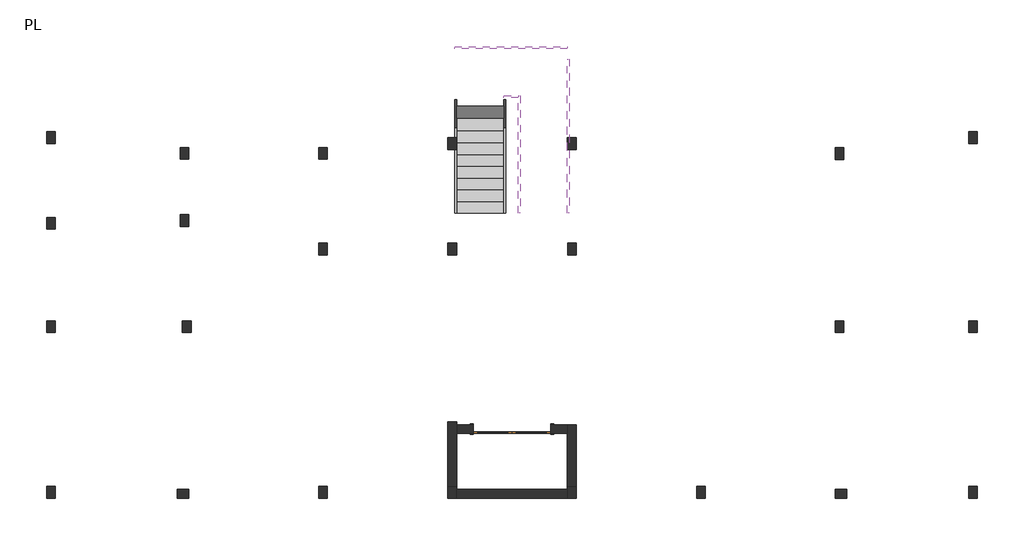
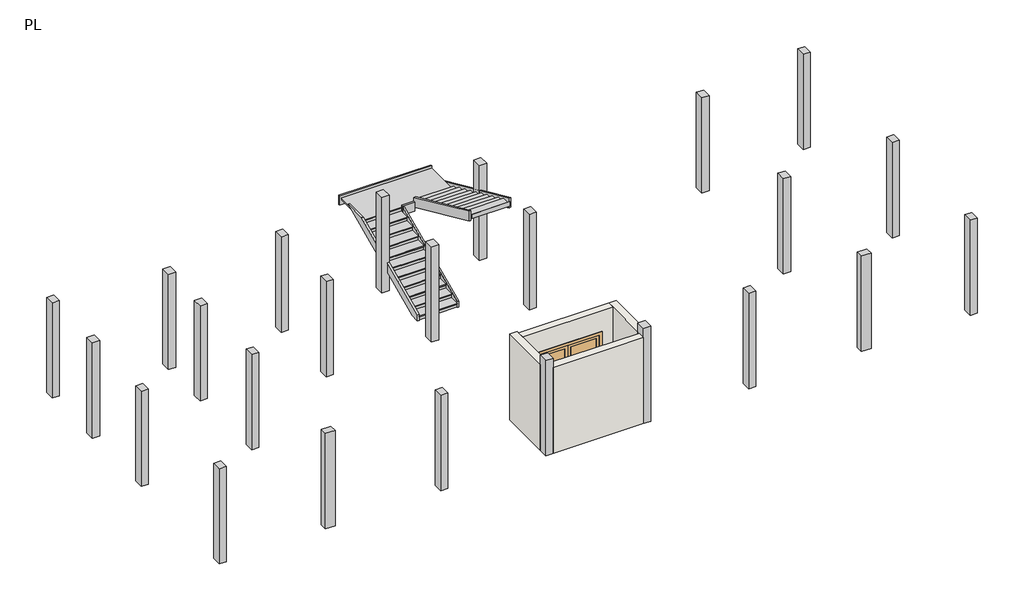
# One storey, incomplete: 24 columns, 6 members, 4 walls, 1 door, 1 stair flight.
"""IFC4 building model written with IfcOpenShell, lengths in millimetres."""

from ifc_helpers import new_model, si_unit, frame, origin, origin_with_axes, place, context, project, spatial, polyline, outline, extrude, faceted_brep, transform, mapped, element, save
from components import column_f87144f2, door_77e2dd85, stair_flight_185d1b01

model = new_model("IFC4")

# Units and contexts
model_context = context("Model", 3, world=origin())
ifc_project = project(units=[si_unit("LENGTHUNIT", "METRE", prefix="MILLI")], contexts=[model_context])

# Site, building, storey
site = spatial("IfcSite", under=ifc_project)
building = spatial("IfcBuilding", under=site)
storey = spatial("IfcBuildingStorey", under=building, Name="PL", Elevation=0.0)

# Columns
placement = place(None, origin())
element("IfcColumn", 1, ObjectType="Rectangular Column : 1'X 9\"", at=placement, inside=storey, context=model_context, shape_type="SweptSolid", body=[
    extrude(outline(polyline([(-12224.6987957, -3709.2932671), (-12224.6987957, -4014.0932671), (-12453.2987957, -4014.0932671), (-12453.2987957, -3709.2932671), (-12224.6987957, -3709.2932671)])), origin_with_axes(), (0.0, 0.0, 1.0), 3200.4),
])
element("IfcColumn", 2, ObjectType="Rectangular Column : 1'X 9\"", at=placement, inside=storey, context=model_context, shape_type="SweptSolid", body=[
    extrude(outline(polyline([(-12224.6987957, 583.3067334), (-12224.6987957, 278.5067334), (-12453.2987957, 278.5067334), (-12453.2987957, 583.3067334), (-12224.6987957, 583.3067334)])), origin_with_axes(), (0.0, 0.0, 1.0), 3200.4),
])
element("IfcColumn", 3, ObjectType="Rectangular Column : 1'X 9\"", at=placement, inside=storey, context=model_context, shape_type="SweptSolid", body=[
    extrude(outline(polyline([(-12224.6987957, 3256.6567332), (-12224.6987957, 2951.8567332), (-12453.2987957, 2951.8567332), (-12453.2987957, 3256.6567332), (-12224.6987957, 3256.6567332)])), origin_with_axes(), (0.0, 0.0, 1.0), 3200.4),
])
element("IfcColumn", 4, ObjectType="Rectangular Column : 1'X 9\"", at=placement, inside=storey, context=model_context, shape_type="SweptSolid", body=[
    extrude(outline(polyline([(-8770.2987992, 5066.406733), (-8770.2987992, 4761.606733), (-8998.8987992, 4761.606733), (-8998.8987992, 5066.406733), (-8770.2987992, 5066.406733)])), origin_with_axes(), (0.0, 0.0, 1.0), 3200.4),
])
element("IfcColumn", 5, ObjectType="Rectangular Column : 1'X 9\"", at=placement, inside=storey, context=model_context, shape_type="SweptSolid", body=[
    extrude(outline(polyline([(-8770.2987992, 3326.5067332), (-8770.2987992, 3021.7067332), (-8998.8987992, 3021.7067332), (-8998.8987992, 3326.5067332), (-8770.2987992, 3326.5067332)])), origin_with_axes(), (0.0, 0.0, 1.0), 3200.4),
])
element("IfcColumn", 6, ObjectType="Rectangular Column : 1'X 9\"", at=placement, inside=storey, context=model_context, shape_type="SweptSolid", body=[
    extrude(outline(polyline([(-8713.148796, 583.3067334), (-8713.148796, 278.5067334), (-8941.748796, 278.5067334), (-8941.748796, 583.3067334), (-8713.148796, 583.3067334)])), origin_with_axes(), (0.0, 0.0, 1.0), 3200.4),
])
element("IfcColumn", 7, ObjectType="Rectangular Column : 1'X 9\"", at=placement, inside=storey, context=model_context, shape_type="SweptSolid", body=[
    extrude(outline(polyline([(-5188.8987995, 5066.406733), (-5188.8987995, 4761.606733), (-5417.4987995, 4761.606733), (-5417.4987995, 5066.406733), (-5188.8987995, 5066.406733)])), origin_with_axes(), (0.0, 0.0, 1.0), 3200.4),
])
element("IfcColumn", 8, ObjectType="Rectangular Column : 1'X 9\"", at=placement, inside=storey, context=model_context, shape_type="SweptSolid", body=[
    extrude(outline(polyline([(-5188.8987995, 2589.9067802), (-5188.8987995, 2285.1067802), (-5417.4987995, 2285.1067802), (-5417.4987995, 2589.9067802), (-5188.8987995, 2589.9067802)])), origin_with_axes(), (0.0, 0.0, 1.0), 3200.4),
])
element("IfcColumn", 9, ObjectType="Rectangular Column : 1'X 9\"", at=placement, inside=storey, context=model_context, shape_type="SweptSolid", body=[
    extrude(outline(polyline([(-5188.8987963, -3709.2932193), (-5188.8987963, -4014.0932193), (-5417.4987963, -4014.0932193), (-5417.4987963, -3709.2932193), (-5188.8987963, -3709.2932193)])), origin_with_axes(), (0.0, 0.0, 1.0), 3200.4),
])
element("IfcColumn", 10, ObjectType="Rectangular Column : 1'X 9\"", at=placement, inside=storey, context=model_context, shape_type="Brep", body=[
    faceted_brep([(1250.0012085, -3709.2932193, 0.0), (1250.0012085, -4014.0932193, 0.0), (1021.4012085, -4014.0932193, 0.0), (1021.4012085, -3785.4932663, 0.0), (1021.4012085, -3709.2932193, 0.0), (1250.0012085, -3709.2932193, 3200.4), (1250.0012085, -4014.0932193, 3200.4), (1250.0012085, -3709.2932193, 2895.6), (1021.4012085, -4014.0932193, 3200.4), (1021.4012085, -3709.2932193, 3200.4), (1021.4012085, -3709.2932193, 2895.6)], [[[0, 1, 2, 3, 4]], [[5, 6, 1, 0, 7]], [[6, 8, 2, 1]], [[8, 9, 10, 4, 3, 2]], [[9, 5, 7, 0, 4, 10]], [[5, 9, 8, 6]]]),
])
element("IfcColumn", 11, ObjectType="Rectangular Column : 1'X 9\"", at=placement, inside=storey, context=model_context, shape_type="SweptSolid", body=[
    extrude(outline(polyline([(4590.1012082, -3709.2932193), (4590.1012082, -4014.0932193), (4361.5012082, -4014.0932193), (4361.5012082, -3709.2932193), (4590.1012082, -3709.2932193)])), origin_with_axes(), (0.0, 0.0, 1.0), 3200.4),
])
element("IfcColumn", 12, ObjectType="Rectangular Column : 1'X 9\"", at=placement, inside=storey, context=model_context, shape_type="SweptSolid", body=[
    extrude(outline(polyline([(11625.9012075, -3709.2932671), (11625.9012075, -4014.0932671), (11397.3012075, -4014.0932671), (11397.3012075, -3709.2932671), (11625.9012075, -3709.2932671)])), origin_with_axes(), (0.0, 0.0, 1.0), 3200.4),
])
element("IfcColumn", 13, ObjectType="Rectangular Column : 1'X 9\"", at=placement, inside=storey, context=model_context, shape_type="SweptSolid", body=[
    extrude(outline(polyline([(11625.9012075, 583.3067295), (11625.9012075, 278.5067295), (11397.3012075, 278.5067295), (11397.3012075, 583.3067295), (11625.9012075, 583.3067295)])), origin_with_axes(), (0.0, 0.0, 1.0), 3200.4),
])
element("IfcColumn", 14, ObjectType="Rectangular Column : 1'X 9\"", at=placement, inside=storey, context=model_context, shape_type="SweptSolid", body=[
    extrude(outline(polyline([(11625.9012075, 5479.1567329), (11625.9012075, 5174.3567329), (11397.3012075, 5174.3567329), (11397.3012075, 5479.1567329), (11625.9012075, 5479.1567329)])), origin_with_axes(), (0.0, 0.0, 1.0), 3200.4),
])
element("IfcColumn", 15, ObjectType="Rectangular Column : 1'X 9\"", at=placement, inside=storey, context=model_context, shape_type="SweptSolid", body=[
    extrude(outline(polyline([(8172.5040565, 5065.4824989), (8172.5040565, 4760.6824989), (7943.9040565, 4760.6824989), (7943.9040565, 5065.4824989), (8172.5040565, 5065.4824989)])), origin_with_axes(), (0.0, 0.0, 1.0), 3200.4),
])
element("IfcColumn", 16, ObjectType="Rectangular Column : 1'X 9\"", at=placement, inside=storey, context=model_context, shape_type="SweptSolid", body=[
    extrude(outline(polyline([(8171.5012047, 583.3067334), (8171.5012047, 278.5067334), (7942.9012047, 278.5067334), (7942.9012047, 583.3067334), (8171.5012047, 583.3067334)])), origin_with_axes(), (0.0, 0.0, 1.0), 3200.4),
])
element("IfcColumn", 17, ObjectType="Rectangular Column : 1'X 9\"", at=placement, inside=storey, context=model_context, shape_type="SweptSolid", body=[
    extrude(outline(polyline([(-9076.550543, -3785.4932196), (-8771.750543, -3785.4932196), (-8771.750543, -4014.0932196), (-9076.550543, -4014.0932196), (-9076.550543, -3785.4932196)])), origin_with_axes(), (0.0, 0.0, 1.0), 3200.4),
])
element("IfcColumn", 18, ObjectType="Rectangular Column : 1'X 9\"", at=placement, inside=storey, context=model_context, shape_type="SweptSolid", body=[
    extrude(outline(polyline([(-12453.2987957, 5174.3567339), (-12453.2987957, 5479.1567339), (-12224.6987957, 5479.1567339), (-12224.6987957, 5174.3567339), (-12453.2987957, 5174.3567339)])), origin_with_axes(), (0.0, 0.0, 1.0), 3200.4),
])
element("IfcColumn", 19, ObjectType="Rectangular Column : 1'X 9\"", at=placement, inside=storey, context=model_context, shape_type="SweptSolid", body=[
    extrude(outline(polyline([(-1845.5417538, 5320.4067329), (-1845.5417538, 5015.6067329), (-2074.1417538, 5015.6067329), (-2074.1417538, 5320.4067329), (-1845.5417538, 5320.4067329)])), origin_with_axes(), (0.0, 0.0, 1.0), 3200.4),
])
element("IfcColumn", 20, ObjectType="Rectangular Column : 1'X 9\"", at=placement, inside=storey, context=model_context, shape_type="SweptSolid", body=[
    extrude(outline(polyline([(1250.0012085, 5320.4067329), (1250.0012085, 5015.6067329), (1021.4012085, 5015.6067329), (1021.4012085, 5320.4067329), (1250.0012085, 5320.4067329)])), origin_with_axes(), (0.0, 0.0, 1.0), 3200.4),
])
element("IfcColumn", 21, ObjectType="Rectangular Column : 1'X 9\"", at=placement, inside=storey, context=model_context, shape_type="SweptSolid", body=[
    extrude(outline(polyline([(-1845.5417538, 2589.906774), (-1845.5417538, 2285.106774), (-2074.1417538, 2285.106774), (-2074.1417538, 2589.906774), (-1845.5417538, 2589.906774)])), origin_with_axes(), (0.0, 0.0, 1.0), 3200.4),
])
element("IfcColumn", 22, ObjectType="Rectangular Column : 1'X 9\"", at=placement, inside=storey, context=model_context, shape_type="SweptSolid", body=[
    extrude(outline(polyline([(1253.2582462, 2589.9067742), (1253.2582462, 2285.1067742), (1024.6582462, 2285.1067742), (1024.6582462, 2589.9067742), (1253.2582462, 2589.9067742)])), origin_with_axes(), (0.0, 0.0, 1.0), 3200.4),
])
element("IfcColumn", 23, ObjectType="Rectangular Column : 1'X 9\"", at=placement, inside=storey, context=model_context, shape_type="Brep", body=[
    faceted_brep([(-1848.7987998, -3709.2932663, 0.0), (-1848.7987998, -3785.4932663, 0.0), (-1848.7987998, -4014.0932663, 0.0), (-2077.3987998, -4014.0932663, 0.0), (-2077.3987998, -3709.2932663, 0.0), (-1848.7987998, -3709.2932663, 3200.4), (-1848.7987998, -4014.0932663, 3200.4), (-1848.7987998, -4014.0932663, 2895.6), (-1848.7987998, -3709.2932663, 2895.6), (-2077.3987998, -4014.0932663, 3200.4), (-2077.3987998, -3709.2932663, 3200.4), (-2077.3987998, -3709.2932663, 2895.6)], [[[0, 1, 2, 3, 4]], [[5, 6, 7, 2, 1, 0, 8]], [[6, 9, 3, 2, 7]], [[9, 10, 11, 4, 3]], [[10, 5, 8, 0, 4, 11]], [[5, 10, 9, 6]]]),
])
column_shape = column_f87144f2(model_context)
element("IfcColumn", 24, ObjectType="Rectangular Column : 1'X 9\"", at=placement, inside=storey, context=model_context, shape_type="MappedRepresentation", body=[
    mapped(column_shape, transform((8094.1646942, -3901.6914801, 0.0), x_axis=(0.0, 1.0, 0.0), y_axis=(-1.0, 0.0, 0.0), z_axis=(0.0, 0.0, 1.0))),
])

# Door
door_shape = door_77e2dd85(model_context)
element("IfcDoor", 25, ObjectType="M_Door-Double-Glass : 6'7\"X7'", at=placement, inside=storey, context=model_context, shape_type="MappedRepresentation", body=[
    mapped(door_shape, transform((-413.6987957, -2221.0120163, 0.0), x_axis=(-1.0, 0.0, 0.0), y_axis=(0.0, -1.0, 0.0), z_axis=(0.0, 0.0, 1.0))),
])

# Members
element("IfcMember", 26, ObjectType="Stringer - 2\" Width", at=placement, inside=storey, context=model_context, shape_type="SweptSolid", body=[
    extrude(outline(polyline([(3364.6067329, 0.0), (3364.6067329, 199.8262721), (6445.4289342, 1600.2), (7182.0114168, 1600.2), (3661.5714168, 0.0), (3364.6067329, 0.0)])), frame((-1896.3417538, 0.0, 0.0), z_axis=(1.0, 0.0, 0.0), x_axis=(0.0, 1.0, 0.0)), (0.0, 0.0, 1.0), 50.8),
])
element("IfcMember", 27, ObjectType="Stringer - 2\" Width", at=placement, inside=storey, context=model_context, shape_type="SweptSolid", body=[
    extrude(outline(polyline([(-1896.3417538, 7631.8067329), (-1896.3417538, 7682.6067329), (1021.4012085, 7682.6067329), (1021.4012085, 7631.8067329), (-1896.3417538, 7631.8067329)])), frame((0.0, 0.0, 1295.4), z_axis=(0.0, 0.0, 1.0), x_axis=(1.0, 0.0, 0.0)), (0.0, 0.0, 1.0), 304.8),
])
element("IfcMember", 28, ObjectType="Stringer - 2\" Width", at=placement, inside=storey, context=model_context, shape_type="SweptSolid", body=[
    extrude(outline(polyline([(6618.562049, 1295.4), (3364.6067329, 2774.4705982), (3364.6067329, 3109.2808176), (7355.1445316, 1295.4), (6618.562049, 1295.4)])), frame((1021.4012085, 0.0, 0.0), z_axis=(1.0, 0.0, 0.0), x_axis=(0.0, 1.0, 0.0)), (0.0, 0.0, 1.0), 50.8),
])
element("IfcMember", 29, ObjectType="Stringer - 2\" Width", at=placement, inside=storey, context=model_context, shape_type="SweptSolid", body=[
    extrude(outline(polyline([(3364.6067329, 0.0), (3364.6067329, 199.8262721), (6361.8067329, 1562.1899085), (6361.8067329, 1227.3796892), (3661.5714168, 0.0), (3364.6067329, 0.0)])), frame((-629.5987998, 0.0, 0.0), z_axis=(1.0, 0.0, 0.0), x_axis=(0.0, 1.0, 0.0)), (0.0, 0.0, 1.0), 50.8),
])
element("IfcMember", 30, ObjectType="Stringer - 2\" Width", at=placement, inside=storey, context=model_context, shape_type="SweptSolid", body=[
    extrude(outline(polyline([(-629.5987998, 6361.8067329), (-629.5987998, 6412.6067329), (-248.5987915, 6412.6067329), (-248.5987915, 6361.8067329), (-629.5987998, 6361.8067329)])), frame((0.0, 0.0, 1295.4), z_axis=(0.0, 0.0, 1.0), x_axis=(1.0, 0.0, 0.0)), (0.0, 0.0, 1.0), 304.8),
])
element("IfcMember", 31, ObjectType="Stringer - 2\" Width", at=placement, inside=storey, context=model_context, shape_type="SweptSolid", body=[
    extrude(outline(polyline([(6412.6067329, 1723.8262721), (6412.6067329, 1389.0160528), (3364.6067329, 2774.4705982), (3364.6067329, 3109.2808176), (6412.6067329, 1723.8262721)])), frame((-248.5987915, 0.0, 0.0), z_axis=(1.0, 0.0, 0.0), x_axis=(0.0, 1.0, 0.0)), (0.0, 0.0, 1.0), 50.8),
])

# Stair flight
stair_flight_shape = stair_flight_185d1b01(model_context)
element("IfcStairFlight", 32, ObjectType="2\" Tread 1\" Nosing 1/4\" Riser", at=placement, inside=storey, context=model_context, shape_type="MappedRepresentation", body=[
    mapped(stair_flight_shape, transform((0.0, 0.0, 0.0), x_axis=(1.0, 0.0, 0.0), y_axis=(0.0, 1.0, 0.0), z_axis=(0.0, 0.0, 1.0))),
])

# Walls
element("IfcWall", 33, ObjectType="9\"", at=placement, inside=storey, context=model_context, shape_type="Brep", body=[
    faceted_brep([(-1848.7987998, -3709.2932663, 0.0), (-1848.7987998, -2337.6932663, 0.0), (-1848.7987998, -2109.0932663, 0.0), (-1848.7987998, -2032.8932663, 0.0), (-1848.7987998, -2032.8932663, 2895.6), (-1848.7987998, -2109.0932663, 2895.6), (-1848.7987998, -2337.6932663, 2895.6), (-1848.7987998, -3709.2932663, 2895.6), (-2077.3987998, -3709.2932663, 0.0), (-2077.3987998, -3709.2932663, 2895.6), (-2077.3987998, -2032.8932663, 2895.6), (-2077.3987998, -2032.8932663, 0.0)], [[[0, 1, 2, 3, 4, 5, 6, 7]], [[8, 9, 10, 11]], [[3, 2, 1, 0, 8, 11]], [[4, 3, 11, 10]], [[0, 7, 9, 8]], [[7, 6, 5, 4, 10, 9]]]),
])
element("IfcWall", 34, ObjectType="9\"", at=placement, inside=storey, context=model_context, shape_type="SweptSolid", body=[
    extrude(outline(polyline([(0.0, -1848.7987998), (0.0, -1416.9987957), (2133.6, -1416.9987957), (2133.6, 589.6012043), (0.0, 589.6012043), (0.0, 1021.4012085), (2895.6, 1021.4012085), (2895.6, -1848.7987998), (0.0, -1848.7987998)])), frame((0.0, -2337.6932663, 0.0), z_axis=(0.0, 1.0, 0.0), x_axis=(0.0, 0.0, 1.0)), (0.0, 0.0, 1.0), 228.6),
])
element("IfcWall", 35, ObjectType="9\"", at=placement, inside=storey, context=model_context, shape_type="Brep", body=[
    faceted_brep([(1021.4012085, -2109.0932663, 0.0), (1021.4012085, -2337.6932663, 0.0), (1021.4012085, -3709.2932193, 0.0), (1021.4012085, -3709.2932193, 2895.6), (1021.4012085, -2337.6932663, 2895.6), (1021.4012085, -2109.0932663, 2895.6), (1250.0012085, -2109.0932663, 0.0), (1250.0012085, -2109.0932663, 2895.6), (1250.0012085, -3709.2932193, 2895.6), (1250.0012085, -3709.2932193, 0.0)], [[[0, 1, 2, 3, 4, 5]], [[6, 7, 8, 9]], [[2, 1, 0, 6, 9]], [[3, 2, 9, 8]], [[0, 5, 7, 6]], [[5, 4, 3, 8, 7]]]),
])
element("IfcWall", 36, ObjectType="9\"", at=placement, inside=storey, context=model_context, shape_type="SweptSolid", body=[
    extrude(outline(polyline([(1021.4012085, -4014.0932663), (-1848.7987998, -4014.0932663), (-1848.7987998, -3785.4932663), (1021.4012085, -3785.4932663), (1021.4012085, -4014.0932663)])), origin_with_axes(), (0.0, 0.0, 1.0), 2895.6),
])

save(model, "model.ifc")

# Revit data of these elements
# Type "Rectangular Column : 1'X 9\""
#   Assembly Code = "B1010200"
#   Depth = 1' - 0"
#   Offset Base = 0' - 0"
#   Offset Top = 0' - 0"
#   Width = 0' - 9"
#   Material = none
# Type "M_Door-Double-Glass : 6'7\"X7'"
#   Type Mark = "16"
#   Construction Type Id = "opn-d45"
#   Assembly Code = "C1020"
#   Analytic Construction = "Wood frame, double glass door "
#   W = 3' - 3 1/2"
#   Thickness = 0' - 1.9685"
#   Thermal Resistance (R) = 1.8150 (h·ft²·°F)/BTU
#   Swing Angle [instance default] = 90.00°
#   Heat Transfer Coefficient (U) = 0.5510 BTU/(h·ft²·°F)
#   Height = 7' - 0"
#   Bottom Rail = 0' - 3.93701"
#   Top Rail = 0' - 3.93701"
#   Stiles = 0' - 3.93701"
#   Trim Projection = 0' - 0.98425"
#   Trim Width = 0' - 3.14961"
#   Width = 6' - 7"
#   Define Thermal Properties by = 1
#   Glazing = Glass
#   Panel Material = Wood - Birch - Solid Stained Light Low Gloss
#   Trim Material = Paint - Sienna
#   Visual Light Transmittance = 0
#   Solar Heat Gain Coefficient = 0
#   Function = (empty or 0)
#   Wall Closure = (empty or 0)
# Type "9\""
#   Assembly Code = "B2010"
#   Layers, outside or top first: 0' - 9" no material (function 1)
# Elements 1, 2, 3, 4, 5, 6, 7, 8, 9, 11, 12, 13, 14, 15, 16, 17, 18, 19, 20, 21, 22, 24 (IfcColumn, "Rectangular Column : 1'X 9\"")
#   Phase Created = New Construction
# Elements 10, 23 (IfcColumn, "Rectangular Column : 1'X 9\"")
#   Phase Created = New Construction
#   Materials on its faces: "Default Wall"
# Element 25 (IfcDoor, "M_Door-Double-Glass : 6'7\"X7'")
#   Swing Angle = 90.00°
#   Phase Created = New Construction
#   Materials on its faces: "Wood - Birch - Solid Stained Light Low Gloss", "Paint - Sienna", "Glass"
# Elements 26, 27, 28, 29, 30, 31 (IfcMember, "Stringer - 2\" Width")
#   Phase Created = New Construction
# Element 32 (IfcStairFlight, "2\" Tread 1\" Nosing 1/4\" Riser")
#   Phase Created = New Construction
# Elements 33, 34, 35, 36 (IfcWall, "9\"")
#   Top Offset = -0' - 6"
#   Base Offset = 0' - 0"
#   wall height = 9' - 6"
#   Phase Created = New Construction
#   Base Constraint = PL
#   Top Constraint = GL
#   Materials on its faces: "Default Wall"
# Materials
#   "Glass": class "Glass", colour RGB 0 128 192, transparency 0.75, Description = "Soda Lime Glass", Cost = 0
#   "Wood - Birch - Solid Stained Light Low Gloss": class "Wood", colour RGB 210 159 95, transparency 0, Cost = 0
#   "Paint - Sienna": colour RGB 118 70 51, transparency 0, Cost = 0
#   "Default Wall": colour RGB 128 128 128, transparency 0, Cost = 0
